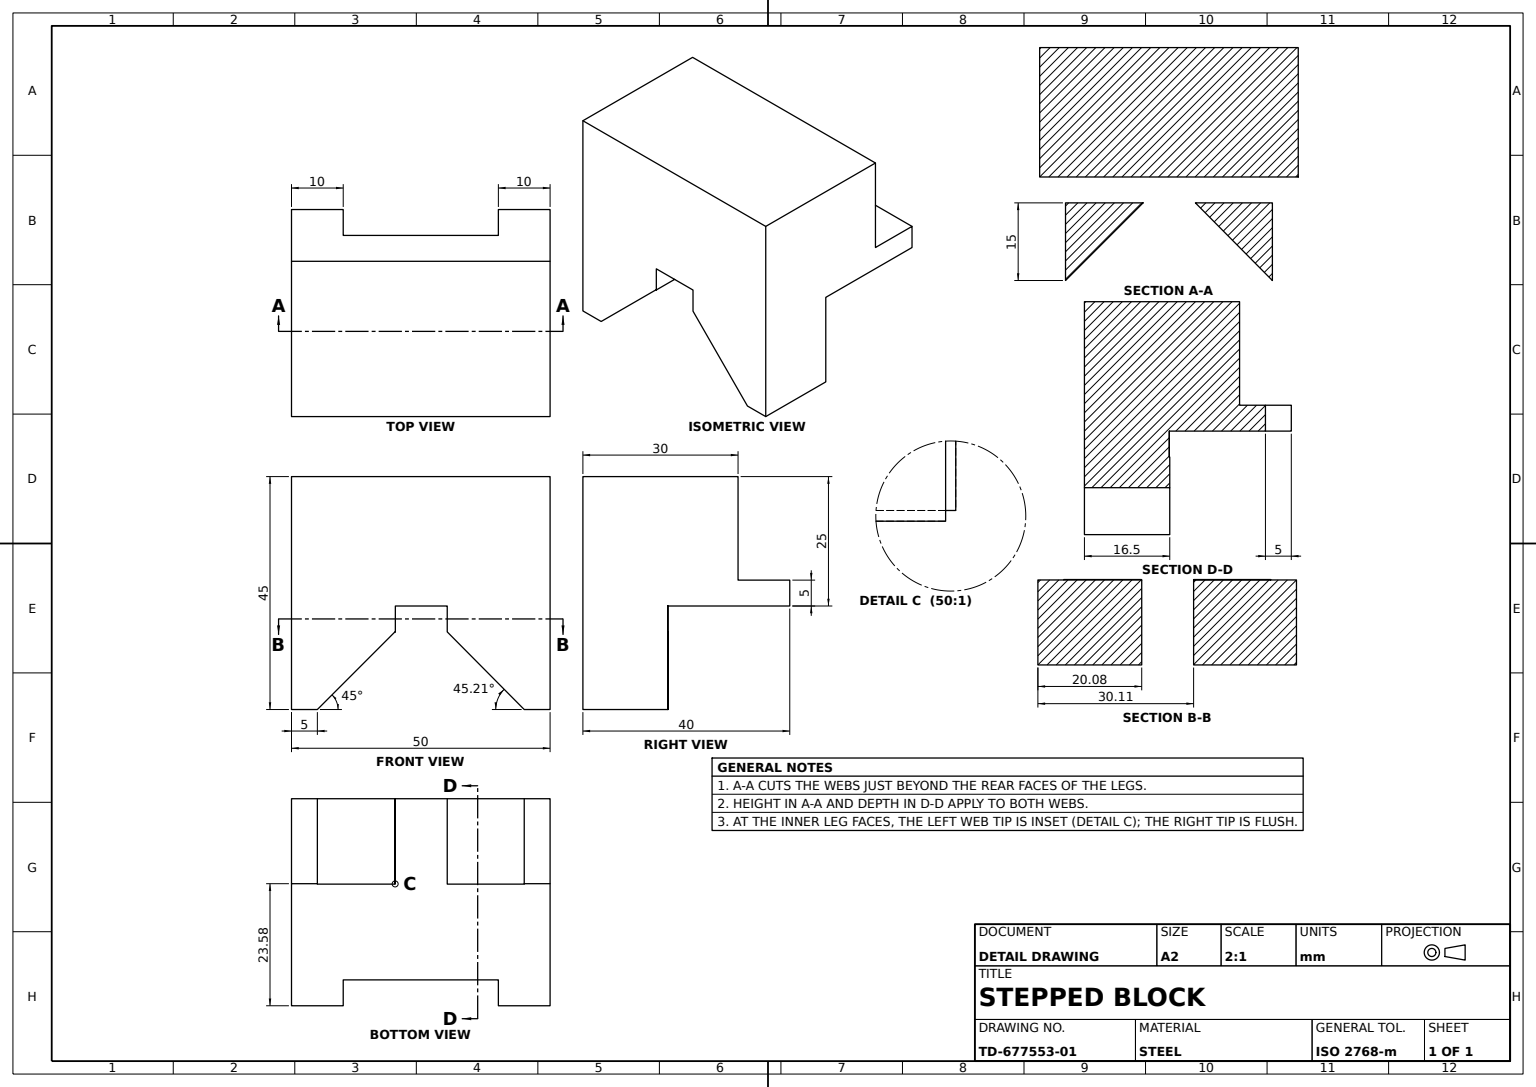
SolidWorks part; units mm, degrees
material "Plain Carbon Steel"
ref_plane "Front Plane" through (0, 0, 0) normal (0, 0, 1) x (1, 0, 0)
ref_plane "Top Plane" through (0, 0, 0) normal (0, 1, 0) x (1, 0, 0)
ref_plane "Right Plane" through (0, 0, 0) normal (1, 0, 0) x (0, 0, -1)
sketch "Base Block Sketch" plane through (0, 0, 0) normal (0, 1, 0) x (1, 0, 0)
  line L1 (0, 0) -> (50, 0)
  line L2 (0, 0) -> (0, 30)
  line L3 (0, 30) -> (50, 30)
  line L4 (50, 0) -> (50, 30)
  dimension "D1" = 50
  dimension "D2" = 30
extrude "Base Block 50x30x25" add sketch "Base Block Sketch" along normal blind 25
sketch "Corner Step Sketch" plane through (0, 0, 0) normal (0, 1, 0) x (1, 0, 0)
  line L0 (0, 30) -> (0, 40)
  line L1 (0, 40) -> (10, 40)
  line L2 (10, 40) -> (10, 35)
  line L3 (10, 35) -> (40, 35)
  line L4 (40, 35) -> (40, 40)
  line L5 (50, 30) -> (50, 40)
  line L6 (50, 40) -> (40, 40)
  line L7 (0, 30) -> (0, 0)
  line L8 (0, 0) -> (50, 0)
  line L9 (50, 0) -> (50, 30)
  line L10 (50, 30) -> (0, 30) construction
  dimension "D1" = 10
  dimension "D2" = 5
  dimension "D3" = 10
  dimension "D4" = 5
  dimension "D5" = 5
  dimension "D6" = 10
  dimension "D7" = 10
extrude "Corner Step 5mm" add sketch "Corner Step Sketch" along normal blind 5
sketch "Lower Plate Sketch" plane through (0, 0, 0) normal (0, -1, 0) x (1, 0, 0)
  line L0 (0, 0) -> (0, -16.4172)
  line L1 (0, -40) -> (0, 0) construction
  line L2 (0, -16.4172) -> (20.0783, -16.4172)
  line L3 (20.0783, -16.4172) -> (20.0783, 0)
  line L4 (0, 0) -> (50, 0) construction
  line L5 (20.0783, 0) -> (0, 0)
  line L6 (20.0783, 0) -> (30.1118, 0)
  line L7 (30.1118, 0) -> (30.1118, -16.4172)
  line L8 (30.1118, -16.4172) -> (20.0783, -16.4172)
  line L9 (30.1118, -16.4172) -> (50, -16.4172)
  line L10 (50, 0) -> (50, -40) construction
  line L11 (50, -16.4172) -> (50, 0)
  line L12 (50, 0) -> (30.1118, 0)
  line L13 (0, 0) -> (6.7707, 0)
  line L14 (10, -40) -> (0, -40) construction
  line L15 (6.7707, -16.4172) -> (0, -16.4172)
  line M1 (0, 0) -> (0, -40)
  line M7 (50, -40) -> (50, 0)
  line M8 (50, 0) -> (0, 0)
  dimension "D1" = 6.7707
  dimension "D2" = 20.0783
  dimension "D3" = 30.1118
  dimension "D4" = 23.5828
extrude "Lower Plate 5mm" add sketch "Lower Plate Sketch" along normal blind 5 contours L2 L3 M8 M1 | L7 L9 M7 M8
sketch "Leg Sketch" plane through (0, -5, 0) normal (0, -1, 0) x (-1, 0, 0)
  line L0 (0, 0) -> (-5, 0)
  line L1 (-20.0783, 0) -> (0, 0) construction
  line L2 (-5, 0) -> (-5, 16.4172)
  line L3 (0, 16.4172) -> (-20.0783, 16.4172) construction
  line L4 (-5, 16.4172) -> (0, 16.4172)
  line L5 (0, 16.4172) -> (0, 0)
  line L6 (-50, 0) -> (-45, 0)
  line L7 (-50, 0) -> (-30.1118, 0) construction
  line L8 (-45, 0) -> (-45, 16.4172)
  line L9 (-30.1118, 16.4172) -> (-50, 16.4172) construction
  line L10 (-45, 16.4172) -> (-50, 16.4172)
  line L11 (-50, 16.4172) -> (-50, 0) construction
  line L12 (-50, 16.4172) -> (-50, 0)
  dimension "D1" = 5
  dimension "D2" = 5
extrude "Leg 15mm" add sketch "Leg Sketch" along normal blind 15
sketch "Tapered Web Direction Line" plane through (0, -20, 0) normal (0, -1, 0) x (-1, 0, 0)
  line L1 (-5, 16.4172) -> (-5, 0)
sketch "Tapered Web Sketch" plane through (0, 0, 0) normal (0, 0, 1) x (1, 0, 0)
  line L0 (30.1118, -5) -> (45, -20)
  line L1 (45, -20) -> (45, -5)
  line L2 (45, -5) -> (30.1118, -5)
  line L3 (5, -5) -> (5, -20)
  line L4 (5, -20) -> (20, -5)
  line L5 (20.0783, -5) -> (5, -5) construction
  line L6 (20, -5) -> (5, -5)
extrude "Tapered Web 16.5mm" add sketch "Tapered Web Sketch" against normal blind 16.5
